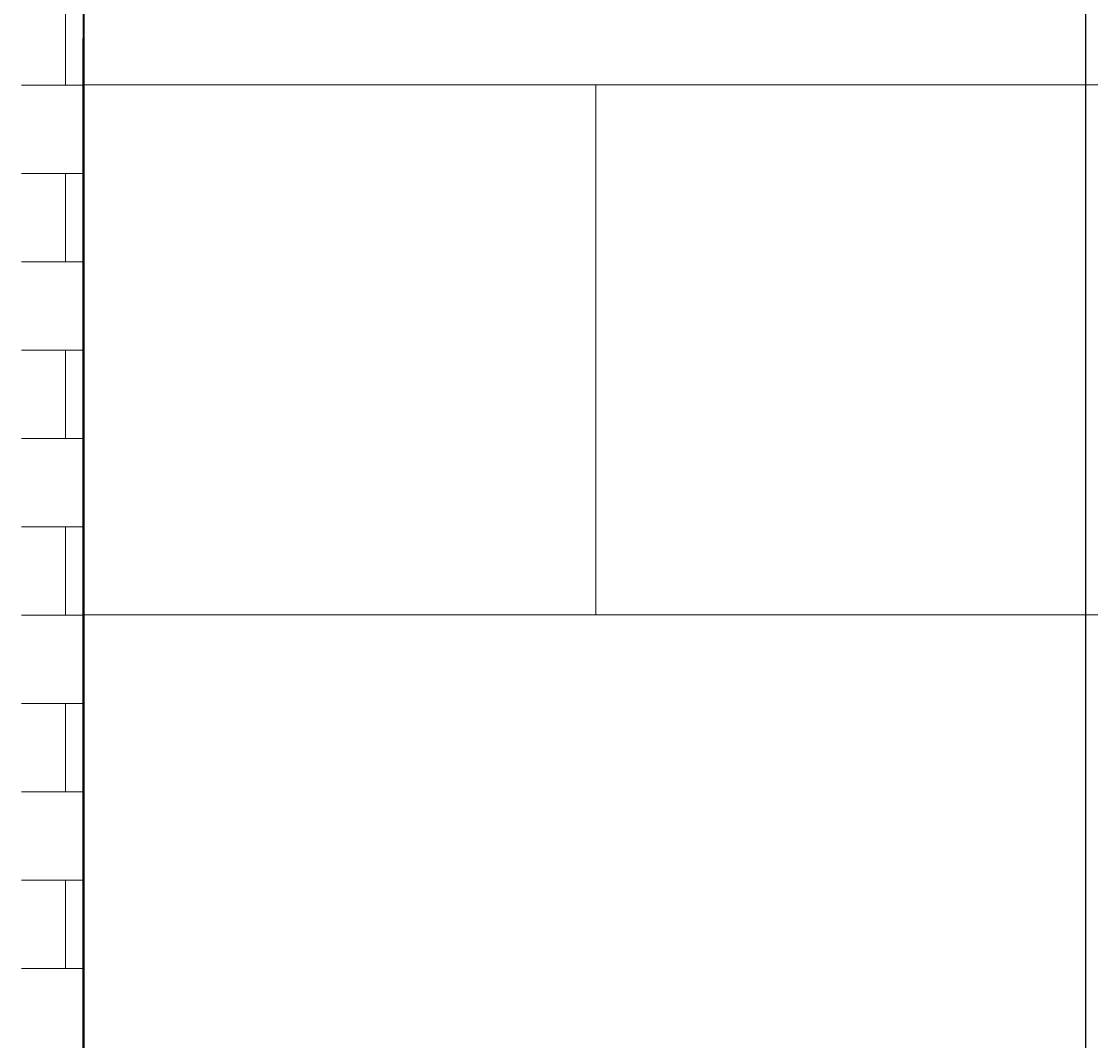
# Model space of a CAD drawing. Units: inches. Extents: x -26 to 776, y -22 to 650.
# Tile 21 of 62: x 285 to 358, y 223 to 292. Entities that reach past the tile are written whole.
import ezdxf

# ---------------------------------------------------------------- set-up
doc = ezdxf.new("R2010")
doc.units = ezdxf.units.IN
doc.header["$MEASUREMENT"] = 0
for name, color, linetype, lineweight in [('A-ANNO-DIMS', 2, 'Continuous', 18), ('A-WALL', 7, 'Continuous', 35), ('A-WALL-PATT', 8, 'Continuous', 13)]:
    doc.layers.add(name, color=color, linetype=linetype, lineweight=lineweight)
doc.styles.get("Standard").update_dxf_attribs({"font": 'arial.ttf'})
doc.dimstyles.get("Standard").update_dxf_attribs({"dimtxt": 0.5625, "dimasz": 0.18, "dimexe": 0.18, "dimexo": 0.0625, "dimgap": 0.09, "dimtad": 0, "dimtih": 1, "dimtoh": 1, "dimdec": 4, "dimzin": 0, "dimdsep": 46, "dimlunit": 4, "dimtxsty": 'Standard', "dimcen": 0.09, "dimadec": 0, "dimazin": 0, "dimtfac": 1, "dimtdec": 4, "dimtofl": 0, "dimtmove": 0, "dimatfit": 3, "dimfxl": 1, "dimtolj": 1, "dimtzin": 0, "dimarcsym": 0})

# ---------------------------------------------------------------- blocks, each defined once
blk = doc.blocks.new('*D28')
at = {"layer": 'A-ANNO-DIMS', "color": 0, "lineweight": -2, "transparency": 16777216}
for p, q in [((285.08, 314.119), (775.335, 314.119)), ((775.155, 313.939), (775.155, 243.141)), ((775.155, 171.597), (775.155, 242.396)), ((285.08, 171.417), (775.335, 171.417))]:
    blk.add_line(p, q, dxfattribs=at)
at = {"layer": 'A-ANNO-DIMS', "color": 0, "transparency": 16777216}
for points in [[(775.125, 313.939), (775.185, 313.939), (775.155, 314.119)], [(775.125, 171.597), (775.185, 171.597), (775.155, 171.417)]]:
    blk.add_solid(points, dxfattribs=at)
at = {"layer": 'Defpoints', "color": 0, "transparency": 16777216}
for p in [(285.018, 314.119), (775.155, 314.119), (285.018, 171.417)]:
    blk.add_point(p, dxfattribs=at)
at = {"layer": 'A-ANNO-DIMS', "color": 0, "transparency": 16777216, "insert": (775.155, 242.768), "char_height": 0.5625, "attachment_point": 5}
blk.add_mtext('\\A1;142.7', dxfattribs=at)
blk = doc.blocks.new('*D34')
at = {"layer": 'A-ANNO-DIMS', "color": 0, "lineweight": -2, "transparency": 16777216}
for p, q in [((228.573, 528.296), (228.573, -21.315)), ((357.303, 528.361), (357.303, -21.315)), ((228.753, -21.135), (291.707, -21.135)), ((357.123, -21.135), (294.17, -21.135))]:
    blk.add_line(p, q, dxfattribs=at)
at = {"layer": 'A-ANNO-DIMS', "color": 0, "transparency": 16777216}
for points in [[(228.753, -21.105), (228.753, -21.165), (228.573, -21.135)], [(357.123, -21.105), (357.123, -21.165), (357.303, -21.135)]]:
    blk.add_solid(points, dxfattribs=at)
at = {"layer": 'Defpoints', "color": 0, "transparency": 16777216}
for p in [(228.573, 528.358), (357.303, 528.423), (357.303, -21.135)]:
    blk.add_point(p, dxfattribs=at)
at = {"layer": 'A-ANNO-DIMS', "color": 0, "transparency": 16777216, "insert": (292.938, -21.135), "char_height": 0.5625, "attachment_point": 5}
blk.add_mtext('\\A1;128.73', dxfattribs=at)
blk = doc.blocks.new('*D39')
at = {"layer": 'A-ANNO-DIMS', "color": 0, "lineweight": -2, "transparency": 16777216}
for p, q in [((289.242, 15.545), (289.242, 649.856)), ((289.422, 649.676), (356.478, 649.676)), ((425.563, 649.676), (358.508, 649.676)), ((425.743, 15.545), (425.743, 649.856))]:
    blk.add_line(p, q, dxfattribs=at)
at = {"layer": 'A-ANNO-DIMS', "color": 0, "transparency": 16777216}
for points in [[(289.422, 649.706), (289.422, 649.646), (289.242, 649.676)], [(425.563, 649.706), (425.563, 649.646), (425.743, 649.676)]]:
    blk.add_solid(points, dxfattribs=at)
at = {"layer": 'Defpoints', "color": 0, "transparency": 16777216}
for p in [(425.743, 649.676), (289.242, 15.482), (425.743, 15.482)]:
    blk.add_point(p, dxfattribs=at)
at = {"layer": 'A-ANNO-DIMS', "color": 0, "transparency": 16777216, "insert": (357.493, 649.676), "char_height": 0.5625, "attachment_point": 5}
blk.add_mtext('\\A1;136.5', dxfattribs=at)

msp = doc.modelspace()

# ---------------------------------------------------------------- hatches: boundary and pattern name
at = {"layer": 'A-WALL-PATT'}
h = msp.add_hatch(dxfattribs=at)
h.set_pattern_fill('AR-B816', color=256, scale=0.75)
h.paths.add_polyline_path([(289.2424, 504.4205), (231.4249, 504.4205), (231.4249, 458.1203), (231.4249, 221.6413), (231.4249, 209.6413), (231.4249, 159.4824), (285.0179, 159.4824), (285.0179, 171.4173), (236.4647, 171.4173), (236.4647, 294.4171), (236.4647, 303.3046), (285.0179, 303.3046), (285.0179, 294.4171), (285.0179, 171.4173), (285.0179, 159.4824), (289.2424, 159.4824), (289.2424, 291.1798), (289.2424, 458.1203)])
h.paths.add_polyline_path([(285.0179, 446.0063), (285.0179, 437.1188), (285.0179, 314.119), (236.4647, 314.119), (236.4647, 437.1188), (236.4647, 446.0063)], flags=16)
h = msp.add_hatch(dxfattribs=at)
h.set_pattern_fill('AR-B816', color=256, scale=4.5)
h.paths.add_polyline_path([(425.7434, 448.2114), (289.2424, 496.9554), (289.2424, 458.1203), (289.2424, 291.1798), (289.2424, 20.7937), (425.7434, 20.7937), (425.7434, 283.2492)])

# ---------------------------------------------------------------- linework, layer by layer
at = {"layer": 'A-WALL'}
for p, q in [((289.2424, 458.1203), (289.2424, 291.1798)), ((289.2424, 159.4824), (289.2424, 291.1798)), ((289.2424, 291.1798), (289.2424, 15.4824))]:
    msp.add_line(p, q, dxfattribs=at)

# ---------------------------------------------------------------- dimensions: what is measured, and where the dimension line sits
at = {"layer": 'A-ANNO-DIMS'}
for base, p1, p2, override, picture, middle in [((425.7434, 649.6763), (289.2424, 15.4824), (425.7434, 15.4824), {"dimdec": 1, "dimlfac": 1, "dimrnd": 0, "dimzin": 0, "dimdsep": 46, "dimlunit": 2}, '*D39', (357.4929, 649.6763)), ((357.3034, -21.1349), (228.5733, 528.3585), (357.3034, 528.4233), {"dimdec": 2, "dimlfac": 1, "dimrnd": 0, "dimzin": 0, "dimdsep": 46, "dimlunit": 2}, '*D34', (292.9384, -21.1349))]:
    dim = msp.add_linear_dim(base=base, p1=p1, p2=p2, dimstyle='Standard', override=override, dxfattribs=at)
    dim.commit()
    dim.dimension.update_dxf_attribs({"geometry": picture, "text_midpoint": middle})
dim = msp.add_linear_dim(base=(775.1553, 314.119), p1=(285.0179, 171.4173), p2=(285.0179, 314.119), angle=90, dimstyle='Standard', override={"dimdec": 1, "dimlfac": 1, "dimrnd": 0, "dimzin": 0, "dimdsep": 46, "dimlunit": 2}, dxfattribs=at)
dim.commit()
dim.dimension.update_dxf_attribs({"geometry": '*D28', "text_midpoint": (775.1553, 242.7682)})

doc.saveas('drawing.dxf')
